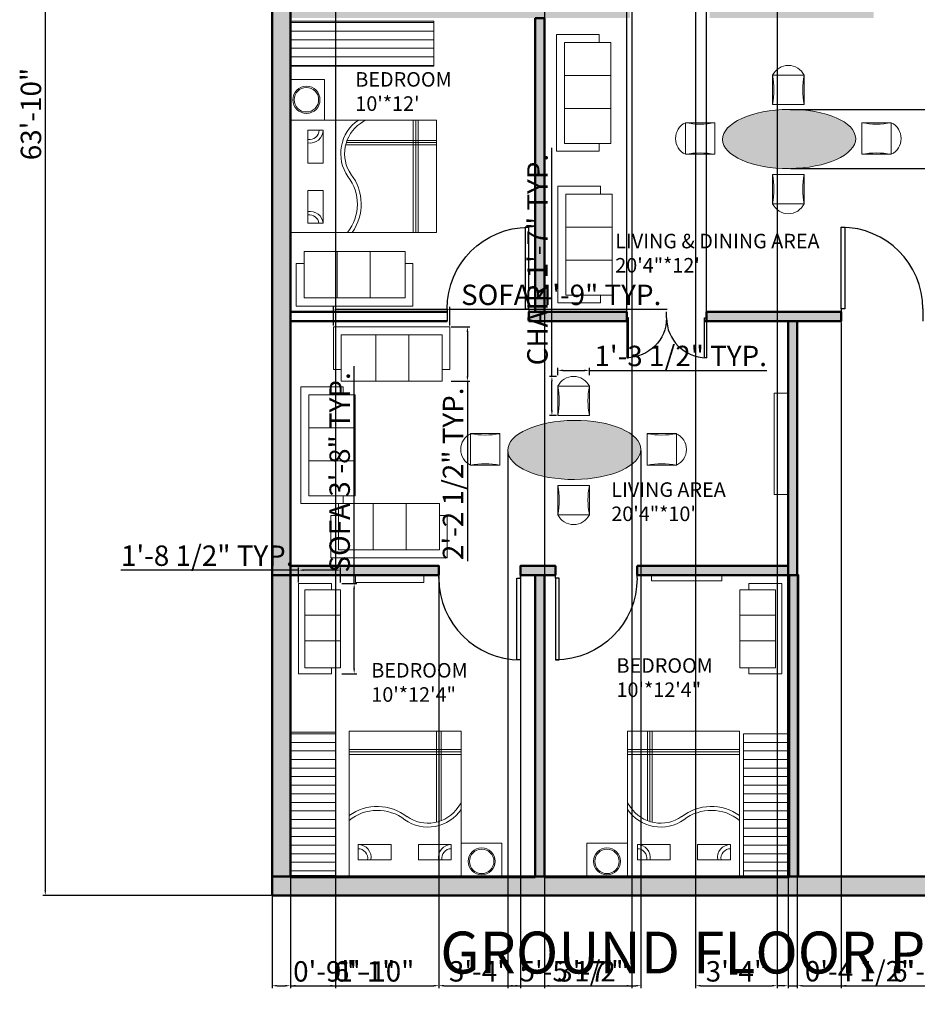
# Model space of a CAD drawing. Units: inches. Extents: x 1477 to 2233, y 1388 to 2326.
# Tile 1 of 4: x 1477 to 1917, y 1388 to 1870. Entities that reach past the tile are written whole.
import ezdxf

# ---------------------------------------------------------------- set-up
doc = ezdxf.new("R2010")
doc.units = ezdxf.units.IN
for name, color, linetype, lineweight in [('A-ANNO-DIMS', 2, 'Continuous', 18), ('A-ANNO-TEXT', 7, 'Continuous', 35), ('A-AREA-IDEN', 7, 'Continuous', 18), ('A-DOOR', 4, 'Continuous', 25), ('A-EQPM', 8, 'Continuous', 18), ('A-FURN-PATT', 9, 'Continuous', 13), ('A-WALL-PATT', 10, 'Continuous', 13), ('bed', 200, 'Continuous', 18), ('book', 104, 'Continuous', 18), ('dining', 220, 'Continuous', 18), ('sofa', 130, 'Continuous', 18), ('table', 40, 'Continuous', 18), ('wall', 10, 'Continuous', 50)]:
    doc.layers.add(name, color=color, linetype=linetype, lineweight=lineweight)
doc.styles.get("Standard").update_dxf_attribs({"font": 'arial.ttf'})
doc.dimstyles.new('ISO-25', dxfattribs={"dimtxt": 10, "dimasz": 2.5, "dimexe": 1.25, "dimexo": 0.625, "dimtad": 1, "dimdec": 0, "dimlunit": 4, "dimtxsty": 'Standard', "dimcen": 2.5, "dimadec": 0, "dimazin": 0, "dimtfac": 1, "dimtdec": 0, "dimtmove": 0, "dimatfit": 3, "dimfxl": 1, "dimarcsym": 0})

# ---------------------------------------------------------------- blocks, each defined once
blk = doc.blocks.new('*U2')
for p, q in [((0, 0), (0, -6)), ((40, 0), (40, -6))]:
    blk.add_line(p, q)
blk.add_lwpolyline([(0, 0), (0, 40), (1.75, 40), (1.75, 0)], close=True)
blk.add_arc((0, 0), 40, 0, 90)
blk = doc.blocks.new('*D5')
at = {"layer": 'A-ANNO-DIMS', "color": 0, "lineweight": -2, "transparency": 16777216}
for p, q in [((1600.48, 2207.17), (1488.68, 2207.17)), ((1489.93, 2204.67), (1489.93, 1443.67)), ((1600.48, 1441.17), (1488.68, 1441.17))]:
    blk.add_line(p, q, dxfattribs=at)
at = {"layer": 'A-ANNO-DIMS', "color": 0, "transparency": 16777216}
for points in [[(1489.51, 2204.67), (1490.35, 2204.67), (1489.93, 2207.17)], [(1489.51, 1443.67), (1490.35, 1443.67), (1489.93, 1441.17)]]:
    blk.add_solid(points, dxfattribs=at)
at = {"layer": 'Defpoints', "color": 0, "transparency": 16777216}
for p in [(1601.11, 2207.17), (1489.93, 1441.17), (1601.11, 1441.17)]:
    blk.add_point(p, dxfattribs=at)
at = {"layer": 'A-ANNO-DIMS', "color": 0, "transparency": 16777216, "insert": (1484.2, 1824.17), "char_height": 10, "attachment_point": 5, "rotation": 90}
blk.add_mtext('63\'-10"', dxfattribs=at)
blk = doc.blocks.new('BED-DOUBLE')
for p, q in [((42.9, 44.24), (42.9, 44.54)), ((42.9, 44.24), (42.9, 0)), ((43.98, 44.24), (43.98, 0)), ((45.09, 43.85), (45.09, 0)), ((53.44, 37.23), (54.99, 35.03)), ((0, 11.42), (54.99, 11.42)), ((0, 10.1), (54.99, 10.1)), ((0, 8.97), (54.99, 8.97))]:
    blk.add_line(p, q)
for points in [[(0, 71.61), (54.99, 71.61), (54.99, 0), (0, 0)], [(4.46, 63.01), (20.6, 63.01), (20.6, 55.57), (4.46, 55.57)], [(50.13, 63.01), (34, 63.01), (34, 55.57), (50.13, 55.57)]]:
    blk.add_lwpolyline(points, close=True)
for centre, radius, start, end in [((4.46, 61.93), 6.36, 270, 9.8305), ((4.46, 62.26), 4.68, 270, 9.2541), ((50.13, 61.93), 6.36, 170.1695, 270), ((50.13, 62.26), 4.68, 170.7459, 270), ((13.85, 60.88), 22.1, 231.1871, 307.7214), ((38.65, 27.17), 19.76, 34.2245, 124.798), ((38.65, 27.17), 17.88, 34.2245, 124.798), ((13.85, 60.88), 23.99, 234.7235, 307.7214)]:
    blk.add_arc(centre, radius, start, end)
blk = doc.blocks.new('BED-DOUBLE-ALT')
for p, q in [((8.97, 0), (8.97, 54.99)), ((10.1, 0), (10.1, 54.99)), ((11.42, 0), (11.42, 54.99)), ((37.23, 53.44), (35.03, 54.99)), ((43.85, 45.09), (0, 45.09)), ((44.24, 43.98), (0, 43.98)), ((44.24, 42.9), (0, 42.9)), ((44.24, 42.9), (44.54, 42.9))]:
    blk.add_line(p, q)
for points in [[(71.61, 0), (71.61, 54.99), (0, 54.99), (0, 0)], [(63.01, 50.13), (63.01, 34), (55.57, 34), (55.57, 50.13)], [(63.01, 4.46), (63.01, 20.6), (55.57, 20.6), (55.57, 4.46)]]:
    blk.add_lwpolyline(points, close=True)
for centre, radius, start, end in [((27.17, 38.65), 17.88, 325.202, 55.7755), ((27.17, 38.65), 19.76, 325.202, 55.7755), ((61.93, 50.13), 6.36, 180, 279.8305), ((62.26, 50.13), 4.68, 180, 279.2541), ((60.88, 13.85), 23.99, 142.2786, 215.2765), ((60.88, 13.85), 22.1, 142.2786, 218.8129), ((61.93, 3.93), 6.36, 80.1695, 175.1865), ((62.26, 3.93), 4.68, 80.7459, 173.4549)]:
    blk.add_arc(centre, radius, start, end)
blk = doc.blocks.new('NIGHTSTAND-LAMP')
blk.add_lwpolyline([(0, 16.8), (19.92, 16.8), (19.92, 0), (0, 0)], close=True)
for radius in [6.66, 6]:
    blk.add_circle((10.02, 8.94), radius)
blk = doc.blocks.new('SOFA-COMPACT-ALT')
for p, q in [((0, 4.5), (0, 20.62)), ((0, 20.62), (44.13, 20.62)), ((44.13, 4.5), (44.13, 20.62)), ((16.11, 17.56), (16.11, 0)), ((28.61, 17.56), (28.61, 0)), ((2.91, 4.5), (0, 4.5)), ((1.29, 4.5), (2.91, 4.5)), ((41.13, 4.5), (44.13, 4.5))]:
    blk.add_line(p, q)
blk.add_lwpolyline([(2.91, 0), (2.91, 17.56), (41.13, 17.56), (41.13, 0)], close=True)
blk = doc.blocks.new('SOFA-STANDARD')
for p, q in [((0, 0), (0, 57.14)), ((20.87, 57.14), (0, 57.14)), ((20.87, 53.26), (20.87, 57.14)), ((3.96, 37.04), (26.7, 37.04)), ((3.96, 20.86), (26.7, 20.86)), ((20.87, 1.67), (20.87, 3.76)), ((20.87, 3.76), (20.87, 0)), ((0, 0), (20.87, 0))]:
    blk.add_line(p, q)
blk.add_lwpolyline([(26.7, 3.76), (3.96, 3.76), (3.96, 53.26), (26.7, 53.26)], close=True)
blk = doc.blocks.new('SOFA-STANDARD-ALT')
for p, q in [((0, 26.7), (57.14, 26.7)), ((0, 26.7), (0, 5.83)), ((57.14, 5.83), (57.14, 26.7)), ((20.86, 22.74), (20.86, 0)), ((37.04, 22.74), (37.04, 0)), ((3.76, 5.83), (0, 5.83)), ((53.26, 5.83), (57.14, 5.83))]:
    blk.add_line(p, q)
blk.add_lwpolyline([(3.76, 0), (3.76, 22.74), (53.26, 22.74), (53.26, 0)], close=True)
blk = doc.blocks.new('CHAIR-DINING')
blk.add_lwpolyline([(0, 0), (15.48, 0), (15.48, 14.4), (0, 14.4)], close=True)
for centre, radius, start, end in [((7.74, 10.64), 8.6, 25.8733, 154.1267), ((-38.59, 7.2), 39.26, 349.434, 10.566), ((53.9, 7.2), 39.09, 169.3873, 190.6127)]:
    blk.add_arc(centre, radius, start, end)
blk = doc.blocks.new('*D15')
at = {"layer": 'A-ANNO-DIMS', "color": 0, "lineweight": -2, "transparency": 16777216}
for p, q in [((1738.31, 1695.61), (1738.31, 1807.55)), ((1740.58, 1695.61), (1737.06, 1695.61)), ((1738.31, 1678.87), (1738.31, 1693.11)), ((1740.58, 1676.37), (1737.06, 1676.37))]:
    blk.add_line(p, q, dxfattribs=at)
at = {"layer": 'A-ANNO-DIMS', "color": 0, "transparency": 16777216}
for points in [[(1737.9, 1693.11), (1738.73, 1693.11), (1738.31, 1695.61)], [(1737.9, 1678.87), (1738.73, 1678.87), (1738.31, 1676.37)]]:
    blk.add_solid(points, dxfattribs=at)
at = {"layer": 'Defpoints', "color": 0, "transparency": 16777216}
for p in [(1738.31, 1695.61), (1741.2, 1695.61), (1741.2, 1676.37)]:
    blk.add_point(p, dxfattribs=at)
at = {"layer": 'A-ANNO-DIMS', "color": 0, "transparency": 16777216, "insert": (1732.52, 1752.83), "char_height": 10, "attachment_point": 5, "rotation": 90}
blk.add_mtext('CHAIR 1\'-7" TYP.', dxfattribs=at)
blk = doc.blocks.new('*D16')
at = {"layer": 'A-ANNO-DIMS', "color": 0, "lineweight": -2, "transparency": 16777216}
for p, q in [((1741.2, 1696.24), (1741.2, 1699.75)), ((1756.68, 1696.24), (1756.68, 1699.75)), ((1743.7, 1698.5), (1754.18, 1698.5)), ((1756.68, 1698.5), (1843.74, 1698.5))]:
    blk.add_line(p, q, dxfattribs=at)
at = {"layer": 'A-ANNO-DIMS', "color": 0, "transparency": 16777216}
for points in [[(1743.7, 1698.92), (1743.7, 1698.09), (1741.2, 1698.5)], [(1754.18, 1698.92), (1754.18, 1698.09), (1756.68, 1698.5)]]:
    blk.add_solid(points, dxfattribs=at)
at = {"layer": 'Defpoints', "color": 0, "transparency": 16777216}
for p in [(1741.2, 1695.61), (1756.68, 1698.5), (1756.68, 1695.61)]:
    blk.add_point(p, dxfattribs=at)
at = {"layer": 'A-ANNO-DIMS', "color": 0, "transparency": 16777216, "insert": (1801.46, 1704.3), "char_height": 10, "attachment_point": 5}
blk.add_mtext('1\'-3 1/2" TYP.', dxfattribs=at)
blk = doc.blocks.new('*D21')
at = {"layer": 'A-ANNO-DIMS', "color": 0, "lineweight": -2, "transparency": 16777216}
for p, q in [((1641.36, 1594), (1641.36, 1700.57)), ((1635.37, 1594), (1642.61, 1594)), ((1641.36, 1552.37), (1641.36, 1591.5)), ((1635.37, 1549.87), (1642.61, 1549.87))]:
    blk.add_line(p, q, dxfattribs=at)
at = {"layer": 'A-ANNO-DIMS', "color": 0, "transparency": 16777216}
for points in [[(1640.95, 1591.5), (1641.78, 1591.5), (1641.36, 1594)], [(1640.95, 1552.37), (1641.78, 1552.37), (1641.36, 1549.87)]]:
    blk.add_solid(points, dxfattribs=at)
at = {"layer": 'Defpoints', "color": 0, "transparency": 16777216}
for p in [(1634.74, 1594), (1641.36, 1594), (1634.74, 1549.87)]:
    blk.add_point(p, dxfattribs=at)
at = {"layer": 'A-ANNO-DIMS', "color": 0, "transparency": 16777216, "insert": (1635.56, 1648.54), "char_height": 10, "attachment_point": 5, "rotation": 90}
blk.add_mtext('SOFA 3\'-8" TYP.', dxfattribs=at)
blk = doc.blocks.new('*D22')
at = {"layer": 'A-ANNO-DIMS', "color": 0, "lineweight": -2, "transparency": 16777216}
for p, q in [((1614.12, 1600.62), (1527.05, 1600.62)), ((1614.12, 1594.62), (1614.12, 1601.87)), ((1632.24, 1600.62), (1616.62, 1600.62)), ((1634.74, 1594.62), (1634.74, 1601.87))]:
    blk.add_line(p, q, dxfattribs=at)
at = {"layer": 'A-ANNO-DIMS', "color": 0, "transparency": 16777216}
for points in [[(1616.62, 1601.04), (1616.62, 1600.2), (1614.12, 1600.62)], [(1632.24, 1601.04), (1632.24, 1600.2), (1634.74, 1600.62)]]:
    blk.add_solid(points, dxfattribs=at)
at = {"layer": 'Defpoints', "color": 0, "transparency": 16777216}
for p in [(1614.12, 1600.62), (1614.12, 1594), (1634.74, 1594)]:
    blk.add_point(p, dxfattribs=at)
at = {"layer": 'A-ANNO-DIMS', "color": 0, "transparency": 16777216, "insert": (1569.34, 1606.41), "char_height": 10, "attachment_point": 5}
blk.add_mtext('1\'-8 1/2" TYP.', dxfattribs=at)
blk = doc.blocks.new('*D27')
at = {"layer": 'A-ANNO-DIMS', "color": 0, "lineweight": -2, "transparency": 16777216}
for p, q in [((1631.2, 1720.51), (1631.2, 1729.71)), ((1633.7, 1728.46), (1685.84, 1728.46)), ((1688.34, 1720.51), (1688.34, 1729.71)), ((1688.34, 1728.46), (1794.91, 1728.46))]:
    blk.add_line(p, q, dxfattribs=at)
at = {"layer": 'A-ANNO-DIMS', "color": 0, "transparency": 16777216}
for points in [[(1633.7, 1728.88), (1633.7, 1728.04), (1631.2, 1728.46)], [(1685.84, 1728.88), (1685.84, 1728.04), (1688.34, 1728.46)]]:
    blk.add_solid(points, dxfattribs=at)
at = {"layer": 'Defpoints', "color": 0, "transparency": 16777216}
for p in [(1688.34, 1728.46), (1631.2, 1719.89), (1688.34, 1719.89)]:
    blk.add_point(p, dxfattribs=at)
at = {"layer": 'A-ANNO-DIMS', "color": 0, "transparency": 16777216, "insert": (1742.88, 1734.26), "char_height": 10, "attachment_point": 5}
blk.add_mtext('SOFA 4\'-9" TYP.', dxfattribs=at)
blk = doc.blocks.new('*D28')
at = {"layer": 'A-ANNO-DIMS', "color": 0, "lineweight": -2, "transparency": 16777216}
for p, q in [((1688.96, 1719.89), (1698.16, 1719.89)), ((1696.91, 1717.39), (1696.91, 1695.69)), ((1688.96, 1693.19), (1698.16, 1693.19)), ((1696.91, 1693.19), (1696.91, 1605.01))]:
    blk.add_line(p, q, dxfattribs=at)
at = {"layer": 'A-ANNO-DIMS', "color": 0, "transparency": 16777216}
for points in [[(1696.49, 1717.39), (1697.33, 1717.39), (1696.91, 1719.89)], [(1696.49, 1695.69), (1697.33, 1695.69), (1696.91, 1693.19)]]:
    blk.add_solid(points, dxfattribs=at)
at = {"layer": 'Defpoints', "color": 0, "transparency": 16777216}
for p in [(1688.34, 1719.89), (1688.34, 1693.19), (1696.91, 1693.19)]:
    blk.add_point(p, dxfattribs=at)
at = {"layer": 'A-ANNO-DIMS', "color": 0, "transparency": 16777216, "insert": (1691.11, 1647.85), "char_height": 10, "attachment_point": 5, "rotation": 90}
blk.add_mtext('2\'-2 1/2" TYP.', dxfattribs=at)
blk = doc.blocks.new('*D33')
at = {"layer": 'A-ANNO-DIMS', "color": 0, "lineweight": -2, "transparency": 16777216}
for p, q in [((1880.17, 1722.05), (1880.17, 1395.67)), ((1960.17, 1722.05), (1960.17, 1395.67)), ((1882.67, 1396.92), (1957.67, 1396.92))]:
    blk.add_line(p, q, dxfattribs=at)
at = {"layer": 'A-ANNO-DIMS', "color": 0, "transparency": 16777216}
for points in [[(1882.67, 1397.34), (1882.67, 1396.51), (1880.17, 1396.92)], [(1957.67, 1397.34), (1957.67, 1396.51), (1960.17, 1396.92)]]:
    blk.add_solid(points, dxfattribs=at)
at = {"layer": 'Defpoints', "color": 0, "transparency": 16777216}
for p in [(1880.17, 1722.67), (1960.17, 1722.67), (1960.17, 1396.92)]:
    blk.add_point(p, dxfattribs=at)
at = {"layer": 'A-ANNO-DIMS', "color": 0, "transparency": 16777216, "insert": (1920.17, 1402.65), "char_height": 10, "attachment_point": 5}
blk.add_mtext('6\'-8"', dxfattribs=at)
blk = doc.blocks.new('*D38')
at = {"layer": 'A-ANNO-DIMS', "color": 0, "lineweight": -2, "transparency": 16777216}
for p, q in [((1682.89, 1597.55), (1682.89, 1395.67)), ((1722.89, 1597.55), (1722.89, 1395.67)), ((1685.39, 1396.92), (1720.39, 1396.92))]:
    blk.add_line(p, q, dxfattribs=at)
at = {"layer": 'A-ANNO-DIMS', "color": 0, "transparency": 16777216}
for points in [[(1685.39, 1397.34), (1685.39, 1396.51), (1682.89, 1396.92)], [(1720.39, 1397.34), (1720.39, 1396.51), (1722.89, 1396.92)]]:
    blk.add_solid(points, dxfattribs=at)
at = {"layer": 'Defpoints', "color": 0, "transparency": 16777216}
for p in [(1682.89, 1598.17), (1722.89, 1598.17), (1722.89, 1396.92)]:
    blk.add_point(p, dxfattribs=at)
at = {"layer": 'A-ANNO-DIMS', "color": 0, "transparency": 16777216, "insert": (1702.89, 1402.66), "char_height": 10, "attachment_point": 5}
blk.add_mtext('3\'-4"', dxfattribs=at)
blk = doc.blocks.new('*D39')
at = {"layer": 'A-ANNO-DIMS', "color": 0, "lineweight": -2, "transparency": 16777216}
for p, q in [((1610.11, 1597.55), (1610.11, 1395.67)), ((1682.89, 1597.55), (1682.89, 1395.67)), ((1612.61, 1396.92), (1680.39, 1396.92))]:
    blk.add_line(p, q, dxfattribs=at)
at = {"layer": 'A-ANNO-DIMS', "color": 0, "transparency": 16777216}
for points in [[(1612.61, 1397.34), (1612.61, 1396.51), (1610.11, 1396.92)], [(1680.39, 1397.34), (1680.39, 1396.51), (1682.89, 1396.92)]]:
    blk.add_solid(points, dxfattribs=at)
at = {"layer": 'Defpoints', "color": 0, "transparency": 16777216}
for p in [(1610.11, 1598.17), (1682.89, 1598.17), (1682.89, 1396.92)]:
    blk.add_point(p, dxfattribs=at)
at = {"layer": 'A-ANNO-DIMS', "color": 0, "transparency": 16777216, "insert": (1646.5, 1402.65), "char_height": 10, "attachment_point": 5}
blk.add_mtext('6\'-1"', dxfattribs=at)
blk = doc.blocks.new('*D41')
at = {"layer": 'A-ANNO-DIMS', "color": 0, "lineweight": -2, "transparency": 16777216}
for p, q in [((1610.11, 2126.39), (1610.11, 1395.67)), ((1632.2, 2126.39), (1632.2, 1395.67)), ((1612.61, 1396.92), (1629.7, 1396.92)), ((1632.2, 1396.92), (1669.36, 1396.92))]:
    blk.add_line(p, q, dxfattribs=at)
at = {"layer": 'A-ANNO-DIMS', "color": 0, "transparency": 16777216}
for points in [[(1612.61, 1397.34), (1612.61, 1396.51), (1610.11, 1396.92)], [(1629.7, 1397.34), (1629.7, 1396.51), (1632.2, 1396.92)]]:
    blk.add_solid(points, dxfattribs=at)
at = {"layer": 'Defpoints', "color": 0, "transparency": 16777216}
for p in [(1610.11, 2127.01), (1632.2, 2127.01), (1632.2, 1396.92)]:
    blk.add_point(p, dxfattribs=at)
at = {"layer": 'A-ANNO-DIMS', "color": 0, "transparency": 16777216, "insert": (1652.03, 1402.65), "char_height": 10, "attachment_point": 5}
blk.add_mtext('1\'-10"', dxfattribs=at)
blk = doc.blocks.new('*D43')
at = {"layer": 'A-ANNO-DIMS', "color": 0, "lineweight": -2, "transparency": 16777216}
for p, q in [((1716.65, 1658.66), (1716.65, 1395.67)), ((1781.95, 1659.2), (1781.95, 1395.67)), ((1719.15, 1396.92), (1779.45, 1396.92))]:
    blk.add_line(p, q, dxfattribs=at)
at = {"layer": 'A-ANNO-DIMS', "color": 0, "transparency": 16777216}
for points in [[(1719.15, 1397.34), (1719.15, 1396.51), (1716.65, 1396.92)], [(1779.45, 1397.34), (1779.45, 1396.51), (1781.95, 1396.92)]]:
    blk.add_solid(points, dxfattribs=at)
at = {"layer": 'Defpoints', "color": 0, "transparency": 16777216}
for p in [(1716.65, 1659.28), (1781.95, 1659.82), (1781.95, 1396.92)]:
    blk.add_point(p, dxfattribs=at)
at = {"layer": 'A-ANNO-DIMS', "color": 0, "transparency": 16777216, "insert": (1749.3, 1402.72), "char_height": 10, "attachment_point": 5}
blk.add_mtext('5\'-5 1/2"', dxfattribs=at)
blk = doc.blocks.new('*D44')
at = {"layer": 'A-ANNO-DIMS', "color": 0, "lineweight": -2, "transparency": 16777216}
for p, q in [((1855.11, 1826.44), (2159.11, 1826.44)), ((2157.86, 1799.98), (2157.86, 1823.94)), ((1855.35, 1797.48), (2159.11, 1797.48))]:
    blk.add_line(p, q, dxfattribs=at)
at = {"layer": 'A-ANNO-DIMS', "color": 0, "transparency": 16777216}
for points in [[(2157.44, 1823.94), (2158.27, 1823.94), (2157.86, 1826.44)], [(2157.44, 1799.98), (2158.27, 1799.98), (2157.86, 1797.48)]]:
    blk.add_solid(points, dxfattribs=at)
at = {"layer": 'Defpoints', "color": 0, "transparency": 16777216}
for p in [(1854.49, 1826.44), (2157.86, 1826.44), (1854.73, 1797.48)]:
    blk.add_point(p, dxfattribs=at)
at = {"layer": 'A-ANNO-DIMS', "color": 0, "transparency": 16777216, "insert": (2152.13, 1811.96), "char_height": 10, "attachment_point": 5, "rotation": 90}
blk.add_mtext('2\'-5"', dxfattribs=at)
blk = doc.blocks.new('*D45')
at = {"layer": 'A-ANNO-DIMS', "color": 0, "lineweight": -2, "transparency": 16777216}
for p, q in [((1601.11, 2031.05), (1601.11, 1395.67)), ((1610.11, 2031.05), (1610.11, 1395.67)), ((1603.61, 1396.92), (1607.61, 1396.92)), ((1610.11, 1396.92), (1640.44, 1396.92))]:
    blk.add_line(p, q, dxfattribs=at)
at = {"layer": 'A-ANNO-DIMS', "color": 0, "transparency": 16777216}
for points in [[(1603.61, 1397.34), (1603.61, 1396.51), (1601.11, 1396.92)], [(1607.61, 1397.34), (1607.61, 1396.51), (1610.11, 1396.92)]]:
    blk.add_solid(points, dxfattribs=at)
at = {"layer": 'Defpoints', "color": 0, "transparency": 16777216}
for p in [(1601.11, 2031.67), (1610.11, 2031.67), (1610.11, 1396.92)]:
    blk.add_point(p, dxfattribs=at)
at = {"layer": 'A-ANNO-DIMS', "color": 0, "transparency": 16777216, "insert": (1626.52, 1402.65), "char_height": 10, "attachment_point": 5}
blk.add_mtext('0\'-9"', dxfattribs=at)
blk = doc.blocks.new('*D46')
at = {"layer": 'A-ANNO-DIMS', "color": 0, "lineweight": -2, "transparency": 16777216}
for p, q in [((1854.12, 1597.55), (1854.12, 1395.67)), ((1858.61, 1597.55), (1858.61, 1395.67)), ((1851.62, 1396.92), (1849.12, 1396.92)), ((1854.12, 1396.92), (1858.61, 1396.92)), ((1861.11, 1396.92), (1914.74, 1396.92))]:
    blk.add_line(p, q, dxfattribs=at)
at = {"layer": 'A-ANNO-DIMS', "color": 0, "transparency": 16777216}
for points in [[(1851.62, 1397.34), (1851.62, 1396.51), (1854.12, 1396.92)], [(1861.11, 1397.34), (1861.11, 1396.51), (1858.61, 1396.92)]]:
    blk.add_solid(points, dxfattribs=at)
at = {"layer": 'Defpoints', "color": 0, "transparency": 16777216}
for p in [(1854.12, 1598.17), (1858.61, 1598.17), (1858.61, 1396.92)]:
    blk.add_point(p, dxfattribs=at)
at = {"layer": 'A-ANNO-DIMS', "color": 0, "transparency": 16777216, "insert": (1889.17, 1402.72), "char_height": 10, "attachment_point": 5}
blk.add_mtext('0\'-4 1/2"', dxfattribs=at)
blk = doc.blocks.new('*D47')
at = {"layer": 'A-ANNO-DIMS', "color": 0, "lineweight": -2, "transparency": 16777216}
for p, q in [((1775, 1723.3), (1775, 2252.67)), ((1777.5, 2251.42), (1811.54, 2251.42)), ((1814.04, 1723.3), (1814.04, 2252.67))]:
    blk.add_line(p, q, dxfattribs=at)
at = {"layer": 'A-ANNO-DIMS', "color": 0, "transparency": 16777216}
for points in [[(1777.5, 2251.84), (1777.5, 2251.01), (1775, 2251.42)], [(1811.54, 2251.84), (1811.54, 2251.01), (1814.04, 2251.42)]]:
    blk.add_solid(points, dxfattribs=at)
at = {"layer": 'Defpoints', "color": 0, "transparency": 16777216}
for p in [(1814.04, 2251.42), (1775, 1722.67), (1814.04, 1722.67)]:
    blk.add_point(p, dxfattribs=at)
at = {"layer": 'A-ANNO-DIMS', "color": 0, "transparency": 16777216, "insert": (1794.52, 2257.16), "char_height": 10, "attachment_point": 5}
blk.add_mtext('3\'-3"', dxfattribs=at)
blk = doc.blocks.new('*D48')
at = {"layer": 'A-ANNO-DIMS', "color": 0, "lineweight": -2, "transparency": 16777216}
for p, q in [((1734.61, 1875.05), (1734.61, 1395.67)), ((1777.43, 1875.05), (1777.43, 1395.67)), ((1737.11, 1396.92), (1774.93, 1396.92))]:
    blk.add_line(p, q, dxfattribs=at)
at = {"layer": 'A-ANNO-DIMS', "color": 0, "transparency": 16777216}
for points in [[(1737.11, 1397.34), (1737.11, 1396.51), (1734.61, 1396.92)], [(1774.93, 1397.34), (1774.93, 1396.51), (1777.43, 1396.92)]]:
    blk.add_solid(points, dxfattribs=at)
at = {"layer": 'Defpoints', "color": 0, "transparency": 16777216}
for p in [(1734.61, 1875.67), (1777.43, 1875.67), (1777.43, 1396.92)]:
    blk.add_point(p, dxfattribs=at)
at = {"layer": 'A-ANNO-DIMS', "color": 0, "transparency": 16777216, "insert": (1756.02, 1402.66), "char_height": 10, "attachment_point": 5}
blk.add_mtext('3\'-7"', dxfattribs=at)
blk = doc.blocks.new('*D49')
at = {"layer": 'A-ANNO-DIMS', "color": 0, "lineweight": -2, "transparency": 16777216}
for p, q in [((1808.79, 2077.55), (1808.79, 1395.67)), ((1848.79, 2077.55), (1848.79, 1395.67)), ((1811.29, 1396.92), (1846.29, 1396.92))]:
    blk.add_line(p, q, dxfattribs=at)
at = {"layer": 'A-ANNO-DIMS', "color": 0, "transparency": 16777216}
for points in [[(1811.29, 1397.34), (1811.29, 1396.51), (1808.79, 1396.92)], [(1846.29, 1397.34), (1846.29, 1396.51), (1848.79, 1396.92)]]:
    blk.add_solid(points, dxfattribs=at)
at = {"layer": 'Defpoints', "color": 0, "transparency": 16777216}
for p in [(1808.79, 2078.17), (1848.79, 2078.17), (1848.79, 1396.92)]:
    blk.add_point(p, dxfattribs=at)
at = {"layer": 'A-ANNO-DIMS', "color": 0, "transparency": 16777216, "insert": (1828.79, 1402.66), "char_height": 10, "attachment_point": 5}
blk.add_mtext('3\'-4"', dxfattribs=at)

msp = doc.modelspace()

# ---------------------------------------------------------------- hatches: boundary and pattern name
at = {"layer": 'A-FURN-PATT'}
h = msp.add_hatch(dxfattribs=at)
h.set_pattern_fill('_USER', color=256, scale=4.2, pattern_type=0)
h.set_pattern_definition([(0, (0, 0), (0, 4.2), [])])
h.paths.add_polyline_path([(1632.2, 2197.32), (1610.11, 2197.32), (1610.11, 2127.01), (1632.2, 2127.01)])
h.paths.add_polyline_path([(1757.03, 2198.17), (1734.93, 2198.17), (1734.93, 2127.87), (1757.03, 2127.87)])
h.paths.add_polyline_path([(1979.11, 2198.17), (1957.06, 2198.17), (1957.06, 2127.87), (1979.11, 2127.87)])
h.paths.add_polyline_path([(2104.61, 2198.17), (2082.56, 2198.17), (2082.56, 2127.87), (2104.61, 2127.87)])
h.paths.add_polyline_path([(2104.61, 1897.77), (2034.3, 1897.77), (2034.3, 1875.67), (2104.61, 1875.67)])
h.paths.add_polyline_path([(1680.41, 1898.15), (1610.11, 1898.15), (1610.11, 1876.06), (1680.41, 1876.06)])
h.paths.add_polyline_path([(1680.41, 1869.67), (1610.11, 1869.67), (1610.11, 1847.57), (1680.41, 1847.57)])
h.paths.add_polyline_path([(1632.2, 1521.19), (1610.11, 1521.19), (1610.11, 1450.88), (1632.2, 1450.88)])
h.paths.add_polyline_path([(1854.34, 1520.43), (1832.24, 1520.43), (1832.24, 1450.17), (1854.34, 1450.17)])
h = msp.add_hatch(color=256, dxfattribs=at)
h.dxf.hatch_style = 1
edge = h.paths.add_edge_path()
edge.add_ellipse((1794.61, 1999.29), major_axis=(32.65, 0.27), ratio=0.443592, start_angle=0, end_angle=360)
edge = h.paths.add_edge_path()
edge.add_ellipse((1920.72, 2000.93), major_axis=(32.65, 0.27), ratio=0.443592, start_angle=0, end_angle=360)
edge = h.paths.add_edge_path()
edge.add_ellipse((1854.61, 1811.96), major_axis=(32.65, 0.27), ratio=0.443592, start_angle=0, end_angle=360)
edge = h.paths.add_edge_path()
edge.add_ellipse((1749.3, 1659.55), major_axis=(32.65, 0.27), ratio=0.443592, start_angle=0, end_angle=360)
at = {"layer": 'A-WALL-PATT'}
h = msp.add_hatch(color=256, dxfattribs=at)
h.dxf.hatch_style = 1
h.paths.add_polyline_path([(2104.61, 2036.17), (1979.11, 2036.17), (1979.11, 2031.67), (2104.61, 2031.67)])
h.paths.add_polyline_path([(1983.61, 2031.67), (1979.11, 2031.67), (1979.11, 2027.53), (1983.61, 2027.53)])
h.paths.add_polyline_path([(1983.61, 2037.7), (1979.11, 2037.7), (1979.11, 2036.17), (1983.61, 2036.17)])
h.paths.add_polyline_path([(2113.61, 2207.17), (2104.61, 2207.17), (2104.61, 2031.67), (2113.61, 2031.67)])
h.paths.add_polyline_path([(2104.61, 2207.17), (1859.11, 2207.17), (1859.11, 2198.17), (2104.61, 2198.17)])
h.paths.add_polyline_path([(1983.61, 2198.17), (1979.16, 2198.17), (1979.16, 2127.87), (1979.11, 2070.31), (1983.61, 2070.31)])
h.paths.add_polyline_path([(1979.11, 2078.17), (1906.33, 2078.17), (1906.33, 2073.67), (1979.11, 2073.67)])
h.paths.add_polyline_path([(1859.11, 2198.17), (1854.61, 2198.17), (1854.61, 2078.17), (1859.11, 2078.17)])
h.paths.add_polyline_path([(1866.33, 2078.17), (1848.79, 2078.17), (1848.79, 2073.67), (1866.33, 2073.67)])
h.paths.add_polyline_path([(1859.11, 2207.17), (1734.61, 2207.17), (1734.61, 2198.17), (1859.11, 2198.17)])
h.paths.add_polyline_path([(1734.61, 2207.17), (1601.11, 2207.17), (1601.11, 2198.17), (1610.11, 2198.17), (1734.61, 2198.17)])
h.paths.add_polyline_path([(1734.61, 2198.17), (1730.11, 2198.17), (1730.11, 2069.66), (1734.61, 2069.66)])
h.paths.add_polyline_path([(1808.79, 2078.17), (1734.61, 2078.17), (1734.61, 2073.67), (1808.79, 2073.67)])
h.paths.add_polyline_path([(1610.11, 2198.17), (1601.11, 2198.17), (1601.11, 1450.43), (1610.11, 1450.43)])
h.paths.add_polyline_path([(2104.61, 1450.43), (1854.61, 1450.43), (1854.61, 1450.17), (1854.34, 1450.13), (1832.24, 1450.13), (1830.34, 1450.13), (1830.34, 1450.03), (1775.35, 1450.03), (1755.43, 1450.03), (1713.79, 1450.14), (1713.79, 1450.03), (1693.87, 1450.03), (1638.87, 1450.03), (1610.11, 1450.17), (1610.11, 1450.43), (1601.11, 1450.43), (1601.11, 1441.17), (2104.61, 1441.17)])
h.paths.add_polyline_path([(2113.61, 1871.17), (2104.61, 1871.17), (2104.61, 1441.17), (2113.61, 1441.17)])
h.paths.add_polyline_path([(1734.61, 1598.17), (1730.11, 1598.17), (1730.11, 1450.43), (1734.61, 1450.43)])
h = msp.add_hatch(color=256, dxfattribs=at)
h.dxf.hatch_style = 1
h.paths.add_polyline_path([(1734.61, 1993.71), (1730.11, 1993.71), (1730.11, 1875.67), (1734.61, 1875.67)])
h.paths.add_polyline_path([(1730.11, 1875.67), (1610.11, 1875.67), (1610.11, 1871.17), (1730.11, 1871.17)])
h.paths.add_polyline_path([(1776.57, 1875.67), (1730.11, 1875.67), (1730.11, 1871.17), (1776.57, 1871.17)])
h.paths.add_polyline_path([(1896.07, 1875.67), (1815.6, 1875.67), (1815.6, 1871.17), (1896.07, 1871.17)])
h.paths.add_polyline_path([(2104.61, 1875.67), (1935.11, 1875.67), (1935.11, 1871.17), (2104.61, 1871.17)])
h.paths.add_polyline_path([(1734.61, 1871.17), (1730.11, 1871.17), (1730.11, 1727.17), (1734.61, 1727.17)])
h.paths.add_polyline_path([(1775, 1727.17), (1726.93, 1727.17), (1726.93, 1722.67), (1775, 1722.67)])
h.paths.add_polyline_path([(1880.17, 1727.17), (1814.04, 1727.17), (1814.04, 1722.67), (1880.17, 1722.67)])
h.paths.add_polyline_path([(1858.61, 1722.67), (1854.11, 1722.67), (1854.12, 1598.17), (1858.61, 1598.17)])
h.paths.add_polyline_path([(1854.12, 1602.67), (1780.08, 1602.67), (1780.08, 1598.17), (1854.12, 1598.17)])
h.paths.add_polyline_path([(1740.08, 1602.67), (1722.89, 1602.67), (1722.89, 1598.17), (1740.08, 1598.17)])
h.paths.add_polyline_path([(1682.89, 1602.67), (1610.11, 1602.67), (1610.11, 1598.17), (1682.89, 1598.17)])
h.paths.add_polyline_path([(1859.11, 1598.17), (1854.61, 1598.17), (1854.61, 1450.43), (1859.11, 1450.43)])
h.paths.add_polyline_path([(2104.61, 1727.17), (1960.17, 1727.17), (1960.17, 1722.67), (2104.61, 1722.67)])
h.paths.add_polyline_path([(2104.61, 1625.03), (1978.61, 1625.03), (1978.61, 1620.53), (2104.61, 1620.53)])

# ---------------------------------------------------------------- linework, layer by layer
at = {"layer": 'A-EQPM'}
for points in [[(1854.11, 1687.3), (1847.26, 1687.3), (1847.26, 1637.63), (1854.11, 1637.63)], [(1642, 1598.17), (1675.57, 1598.17), (1675.57, 1594.54), (1642, 1594.54)], [(1787.18, 1598.17), (1821.64, 1598.17), (1821.64, 1595.38), (1787.18, 1595.38)]]:
    msp.add_lwpolyline(points, close=True, dxfattribs=at)
at = {"layer": 'book'}
for points in [[(1610.11, 1869.67), (1610.11, 1847.57), (1680.41, 1847.57), (1680.41, 1869.67)], [(1632.2, 1450.88), (1610.11, 1450.88), (1610.11, 1521.19), (1632.2, 1521.19)], [(1832.24, 1450.13), (1854.34, 1450.13), (1854.34, 1520.43), (1832.24, 1520.43)]]:
    msp.add_lwpolyline(points, close=True, dxfattribs=at)
at = {"layer": 'dining'}
for centre in [(1854.61, 1811.96), (1749.3, 1659.55)]:
    msp.add_ellipse(centre, major_axis=(32.65, 0.27), ratio=0.443592, dxfattribs=at)
at = {"layer": 'wall'}
for p, q in [((1601.11, 1871.17), (1601.11, 1722.67)), ((1610.11, 1871.17), (1610.11, 1727.17)), ((1730.11, 1727.17), (1730.11, 1871.17)), ((1734.61, 1727.17), (1734.61, 1871.17)), ((1610.11, 1727.17), (1686.93, 1727.17)), ((1730.11, 1727.17), (1726.93, 1727.17)), ((1726.93, 1727.17), (1730.11, 1727.17)), ((1775, 1727.17), (1734.61, 1727.17)), ((1858.61, 1727.17), (1814.04, 1727.17)), ((1858.61, 1727.17), (1880.17, 1727.17)), ((1601.11, 1722.67), (1601.11, 1598.17)), ((1610.11, 1722.67), (1686.93, 1722.67)), ((1610.11, 1722.67), (1610.11, 1602.67)), ((1726.93, 1722.67), (1734.61, 1722.67)), ((1775.86, 1722.67), (1726.93, 1722.67)), ((1794.58, 1722.67), (1794.46, 1722.67)), ((1854.11, 1722.67), (1813.18, 1722.67)), ((1854.11, 1722.67), (1848.66, 1722.67)), ((1854.11, 1602.67), (1854.11, 1722.67)), ((1858.61, 1598.17), (1858.61, 1722.67)), ((1880.17, 1722.67), (1858.61, 1722.67)), ((1610.11, 1602.67), (1682.89, 1602.67)), ((1722.89, 1602.67), (1740.08, 1602.67)), ((1780.08, 1602.67), (1854.11, 1602.67)), ((1601.11, 1598.17), (1682.89, 1598.17)), ((1601.11, 1598.17), (1601.11, 1441.17)), ((1610.11, 1598.17), (1610.11, 1450.17)), ((1722.89, 1598.17), (1740.08, 1598.17)), ((1730.11, 1450.17), (1730.11, 1598.17)), ((1734.61, 1450.17), (1734.61, 1598.17)), ((1734.61, 1598.17), (1740.08, 1598.17)), ((1780.08, 1598.17), (1854.61, 1598.17)), ((1780.08, 1598.17), (1858.61, 1598.17)), ((1854.61, 1598.17), (1854.61, 1450.17)), ((1859.11, 1598.17), (1859.11, 1450.43)), ((1610.11, 1450.17), (1730.11, 1450.17)), ((1854.61, 1450.17), (1734.61, 1450.17)), ((1859.11, 1450.43), (2104.61, 1450.43)), ((1601.11, 1441.17), (1734.61, 1441.17)), ((1859.11, 1441.17), (1734.61, 1441.17)), ((1859.11, 1441.17), (2113.61, 1441.17))]:
    msp.add_line(p, q, dxfattribs=at)
for points in [[(1601.11, 1450.43), (1610.11, 1450.43), (1610.11, 2198.17), (1601.11, 2198.17)], [(1730.11, 1871.17), (1734.61, 1871.17), (1734.61, 1727.17), (1730.11, 1727.17)], [(1726.93, 1722.67), (1775, 1722.67), (1775, 1727.17), (1726.93, 1727.17)], [(1814.04, 1727.17), (1880.17, 1727.17), (1880.17, 1722.67), (1814.04, 1722.67)], [(1854.11, 1722.67), (1858.61, 1722.67), (1858.62, 1598.17), (1854.12, 1598.17)], [(1610.11, 1602.67), (1682.89, 1602.67), (1682.89, 1598.17), (1610.11, 1598.17)], [(1722.89, 1598.17), (1740.08, 1598.17), (1740.08, 1602.67), (1722.89, 1602.67)], [(1780.08, 1602.67), (1854.12, 1602.67), (1854.12, 1598.17), (1780.08, 1598.17)], [(1854.12, 1598.17), (1859.11, 1598.17), (1859.11, 1450.43), (1854.12, 1450.43)], [(2104.61, 1450.43), (1601.11, 1450.43), (1601.11, 1441.17), (2104.61, 1441.17)]]:
    msp.add_lwpolyline(points, close=True, dxfattribs=at)

# ---------------------------------------------------------------- block references
at = {"layer": 'A-DOOR', "xscale": -1}
msp.add_blockref('*U2', (1726.93, 1728.67), dxfattribs=at)
at = {"layer": 'A-DOOR'}
msp.add_blockref('*U2', (1880.17, 1728.67), dxfattribs=at)
at = {"layer": 'A-DOOR', "yscale": 0.4878891377503276, "zscale": 0.4878891377503276, "rotation": 180}
for p, xscale in [((1775, 1724.25), -0.4878891377503276), ((1814.04, 1724.25), 0.4878891377503276)]:
    msp.add_blockref('*U2', p, dxfattribs=dict(at, xscale=xscale))
at = {"layer": 'A-DOOR', "rotation": 180}
msp.add_blockref('*U2', (1722.89, 1596.67), dxfattribs=at)
at = {"layer": 'A-DOOR', "xscale": -1, "rotation": 180}
msp.add_blockref('*U2', (1740.08, 1596.67), dxfattribs=at)
at = {"layer": 'bed', "extrusion": (0, 0, -1), "zscale": -1}
msp.add_blockref('BED-DOUBLE-ALT', (-1681.72, 1766.17), dxfattribs=at)
at = {"layer": 'bed', "extrusion": (0, 0, -1), "zscale": -1, "rotation": 180}
msp.add_blockref('BED-DOUBLE', (-1638.87, 1521.64), dxfattribs=at)
at = {"layer": 'bed', "rotation": 180}
msp.add_blockref('BED-DOUBLE', (1830.34, 1521.64), dxfattribs=at)
at = {"layer": 'dining'}
for p in [(1846.51, 1828.78), (1741.2, 1676.37)]:
    msp.add_blockref('CHAIR-DINING', p, dxfattribs=at)
at = {"layer": 'dining', "extrusion": (0, 0, -1), "zscale": -1}
for p, rotation in [((-1818.17, 1819.92), 269.9999999999994), ((-1846.51, 1794.57), 180), ((-1712.86, 1667.51), 270.0000000000003), ((-1741.2, 1642.16), 180)]:
    msp.add_blockref('CHAIR-DINING', p, dxfattribs=dict(at, rotation=rotation))
at = {"layer": 'dining'}
for p, rotation in [((1890.32, 1819.92), 270.0000000000006), ((1785.01, 1667.51), 270.0000000000003)]:
    msp.add_blockref('CHAIR-DINING', p, dxfattribs=dict(at, rotation=rotation))
at = {"layer": 'sofa'}
for name, p, rotation in [('SOFA-STANDARD-ALT', (1767.25, 1806), 89.99999999999984), ('SOFA-STANDARD-ALT', (1767.91, 1731.69), 89.99999999999808), ('SOFA-STANDARD-ALT', (1670.09, 1756.77), 180), ('SOFA-STANDARD', (1631.2, 1719.89), 270.0000000000011), ('SOFA-COMPACT-ALT', (1634.74, 1549.87), 90.00000000000044)]:
    msp.add_blockref(name, p, dxfattribs=dict(at, rotation=rotation))
msp.add_blockref('SOFA-STANDARD', (1615.17, 1633.3), dxfattribs=at)
at = {"layer": 'sofa', "extrusion": (0, 0, -1), "zscale": -1}
for name, p, rotation in [('SOFA-STANDARD', (-1629.89, 1606.6), 90.00000000000175), ('SOFA-COMPACT-ALT', (-1830.45, 1549.87), 90.00000000000088)]:
    msp.add_blockref(name, p, dxfattribs=dict(at, rotation=rotation))
at = {"layer": 'table'}
for p, rotation in [((1626.9, 1821.16), 89.99999999999923), ((1775.35, 1466.82), 180)]:
    msp.add_blockref('NIGHTSTAND-LAMP', p, dxfattribs=dict(at, rotation=rotation))
at = {"layer": 'table', "extrusion": (0, 0, -1), "zscale": -1, "rotation": 180}
msp.add_blockref('NIGHTSTAND-LAMP', (-1693.87, 1466.82), dxfattribs=at)

# ---------------------------------------------------------------- texts
at = {"layer": 'A-ANNO-TEXT', "insert": (1683.6, 1423.44), "char_height": 20.5255, "attachment_point": 1}
msp.add_mtext_dynamic_manual_height_columns('GROUND FLOOR PLAN', width=2854.7469, gutter_width=102.63, heights=[0], dxfattribs=at)
at = {"layer": 'A-AREA-IDEN', "attachment_point": 1}
for s, insert, char_height in [("BEDROOM\\P10'*12'", (1641.95, 1844.72), 7.116), ('LIVING & DINING AREA\\P20\'4"*12\'', (1769.38, 1765.47), 7.1161), ('LIVING AREA\\P20\'4"*10\'', (1767.44, 1643.65), 7.1161), ('BEDROOM\\P10\'*12\'4"', (1649.79, 1555.08), 7.116), ('BEDROOM\\P10\'*12\'4"', (1769.99, 1557.42), 7.116)]:
    msp.add_mtext_dynamic_manual_height_columns(s, width=109.5726, gutter_width=35.58, heights=[0], dxfattribs=dict(at, insert=insert, char_height=char_height))

# ---------------------------------------------------------------- dimensions: what is measured, and where the dimension line sits
at = {"layer": 'A-ANNO-DIMS'}
for base, p1, p2, picture, middle in [((1814.04, 2251.42), (1775, 1722.67), (1814.04, 1722.67), '*D47', (1794.52, 2257.16)), ((1632.2, 1396.92), (1610.11, 2127.01), (1632.2, 2127.01), '*D41', (1652.03, 1402.65)), ((1848.79, 1396.92), (1808.79, 2078.17), (1848.79, 2078.17), '*D49', (1828.79, 1402.66)), ((1610.11, 1396.92), (1601.11, 2031.67), (1610.11, 2031.67), '*D45', (1626.52, 1402.65)), ((1777.43, 1396.92), (1734.61, 1875.67), (1777.43, 1875.67), '*D48', (1756.02, 1402.66)), ((1960.17, 1396.92), (1880.17, 1722.67), (1960.17, 1722.67), '*D33', (1920.17, 1402.65)), ((1781.95, 1396.92), (1716.65, 1659.28), (1781.95, 1659.82), '*D43', (1749.3, 1402.72)), ((1682.89, 1396.92), (1610.11, 1598.17), (1682.89, 1598.17), '*D39', (1646.5, 1402.65)), ((1722.89, 1396.92), (1682.89, 1598.17), (1722.89, 1598.17), '*D38', (1702.89, 1402.66)), ((1858.61, 1396.92), (1854.12, 1598.17), (1858.61, 1598.17), '*D46', (1889.17, 1402.72))]:
    dim = msp.add_linear_dim(base=base, p1=p1, p2=p2, dimstyle='ISO-25', override={"dimdec": 1, "dimlfac": 1, "dimrnd": 0, "dimzin": 1, "dimdsep": 46, "dimlunit": 4, "dimfrac": 2}, dxfattribs=at)
    dim.commit()
    dim.dimension.update_dxf_attribs({"geometry": picture, "text_midpoint": middle})
for base, p1, p2, override, picture, middle in [((1489.93, 1441.17), (1601.11, 2207.17), (1601.11, 1441.17), {"dimclrd": 0, "dimclre": 0, "dimclrt": 0}, '*D5', (1484.2, 1824.17)), ((2157.86, 1826.44), (1854.73, 1797.48), (1854.49, 1826.44), {"dimdec": 1, "dimlfac": 1, "dimrnd": 0, "dimzin": 1, "dimdsep": 46, "dimlunit": 4, "dimfrac": 2}, '*D44', (2152.13, 1811.96))]:
    dim = msp.add_linear_dim(base=base, p1=p1, p2=p2, angle=90, dimstyle='ISO-25', override=override, dxfattribs=at)
    dim.commit()
    dim.dimension.update_dxf_attribs({"geometry": picture, "text_midpoint": middle})
for base, p1, p2, angle, text, picture, middle in [((1738.31, 1695.61), (1741.2, 1676.37), (1741.2, 1695.61), 90, 'CHAIR <> TYP.', '*D15', (1732.52, 1752.83)), ((1688.34, 1728.46), (1631.2, 1719.89), (1688.34, 1719.89), 0, 'SOFA <> TYP.', '*D27', (1742.88, 1734.26)), ((1696.91, 1693.19), (1688.34, 1719.89), (1688.34, 1693.19), 270, '<> TYP.', '*D28', (1691.11, 1647.85)), ((1641.36, 1594), (1634.74, 1549.87), (1634.74, 1594), 90, 'SOFA <> TYP.', '*D21', (1635.56, 1648.54)), ((1614.12, 1600.62), (1634.74, 1594), (1614.12, 1594), 180, '<> TYP.', '*D22', (1569.34, 1606.41))]:
    dim = msp.add_linear_dim(base=base, p1=p1, p2=p2, angle=angle, text=text, dimstyle='ISO-25', override={"dimdec": 1, "dimlfac": 1, "dimrnd": 0, "dimzin": 1, "dimdsep": 46, "dimlunit": 4, "dimfrac": 2}, dxfattribs=at)
    dim.commit()
    dim.dimension.update_dxf_attribs({"geometry": picture, "text_midpoint": middle})
dim = msp.add_linear_dim(base=(1756.68, 1698.5), p1=(1741.2, 1695.61), p2=(1756.68, 1695.61), text='<> TYP.', dimstyle='ISO-25', override={"dimdec": 1, "dimlfac": 1, "dimrnd": 0, "dimzin": 1, "dimdsep": 46, "dimlunit": 4, "dimfrac": 2}, dxfattribs=at)
dim.commit()
dim.dimension.update_dxf_attribs({"geometry": '*D16', "text_midpoint": (1801.46, 1704.3)})

doc.saveas('drawing.dxf')
